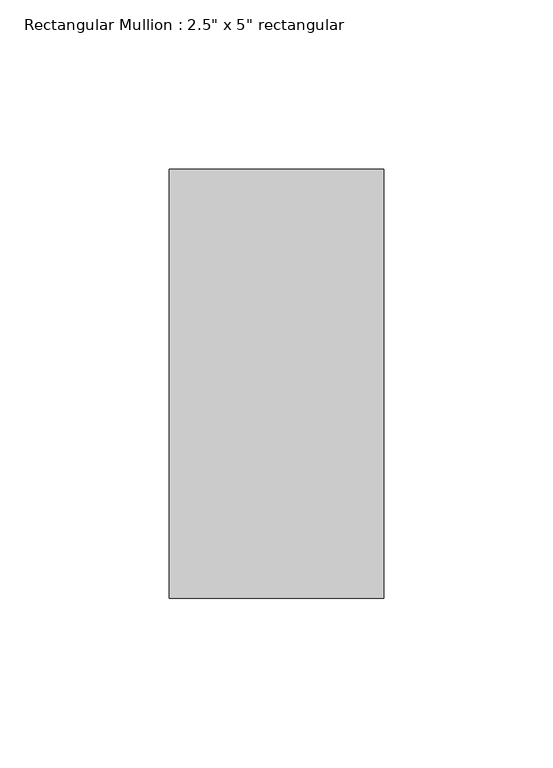
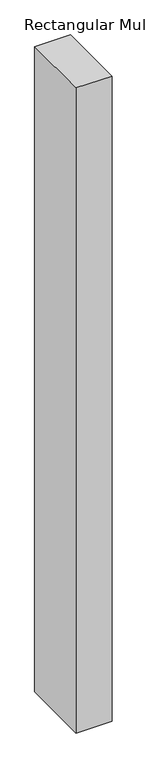
"""IFC4 building model written with IfcOpenShell, lengths in millimetres: member geometry."""

from ifc_helpers import new_model, si_unit, frame, origin, place, context, project, spatial, polyline, outline, extrude, source, transform, mapped, element, save


def member_91edd790(model_context):
    return source(origin(), model_context, "Body", "SweptSolid", [
        extrude(outline(polyline([(0.0, 63.5), (0.0, -63.5), (-63.5, -63.5), (-63.5, 63.5), (0.0, 63.5)])), frame((0.0, 0.0, -1206.4999998), z_axis=(0.0, 0.0, 1.0), x_axis=(1.0, 0.0, 0.0)), (0.0, 0.0, 1.0), 1206.4999998),
    ])


if __name__ == "__main__":
    model = new_model("IFC4")
    model_context = context("Model", 3, world=origin())
    ifc_project = project(units=[si_unit("LENGTHUNIT", "METRE", prefix="MILLI")], contexts=[model_context])
    site = spatial("IfcSite", under=ifc_project)
    building = spatial("IfcBuilding", under=site)
    placement = place(None, origin())
    member_shape = member_91edd790(model_context)
    element("IfcMember", 1, ObjectType="Rectangular Mullion : 2.5\" x 5\" rectangular", at=placement, inside=building, context=model_context, shape_type="MappedRepresentation", body=[
        mapped(member_shape, transform((0.0, 0.0, 0.0), x_axis=(1.0, 0.0, 0.0), y_axis=(0.0, 1.0, 0.0), z_axis=(0.0, 0.0, 1.0))),
    ])
    save(model, "model.ifc")

# Revit data of these elements
# Type "Rectangular Mullion : 2.5\" x 5\" rectangular"
#   built-in parameter 1007304 = 0.416667 (stored number, unit not read)
#   built-in parameter 1007301 = 0.104167 (stored number, unit not read)
#   built-in parameter 1007300 = 0.104167 (stored number, unit not read)
# Element 1 (IfcMember, "Rectangular Mullion : 2.5\" x 5\" rectangular")
#   Materials on its faces: "Aluminum"
# Materials
#   "Aluminum": class "Metal", colour RGB 247 247 247, transparency 0, Description = "Aluminum 6061", Cost = 0
